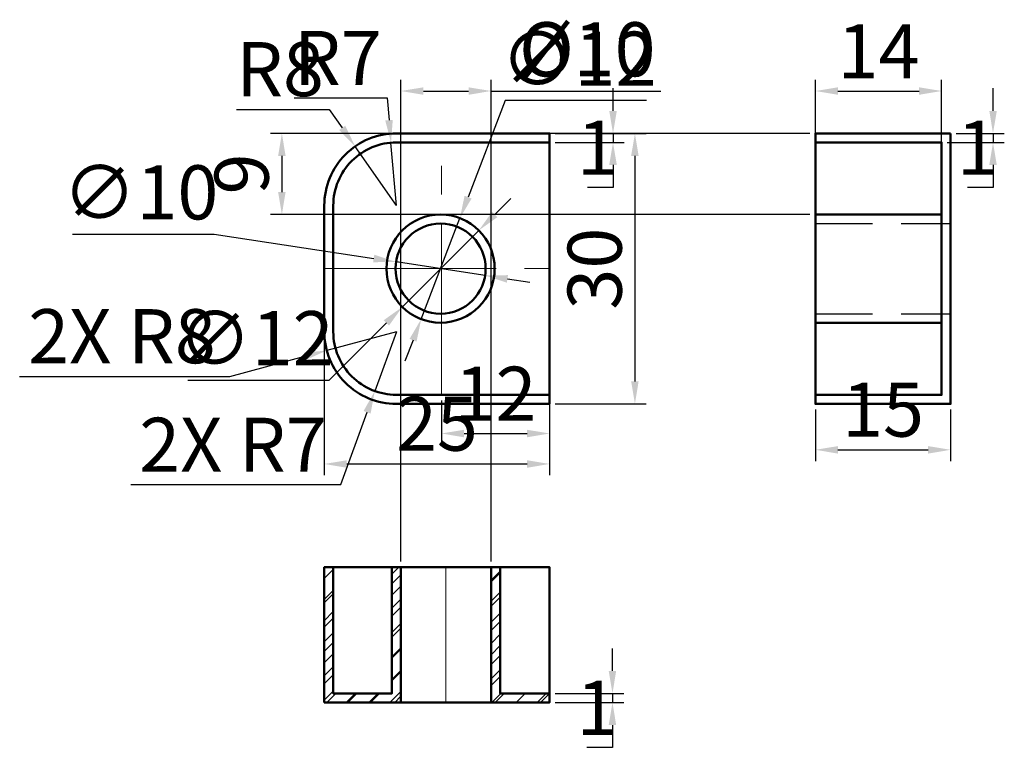
# Model space of a CAD drawing. Units: millimetres. Extents: x 12 to 121, y 26 to 107.
import ezdxf

# ---------------------------------------------------------------- set-up
doc = ezdxf.new("R2010")
doc.units = ezdxf.units.MM
doc.linetypes.add('CENTER2', pattern=[28.575, 19.05, -3.175, 3.175, -3.175])
doc.linetypes.add('HIDDEN', pattern=[9.525, 6.35, -3.175])
for name, color, linetype, lineweight in [('M-CNTR', 1, 'CENTER2', 18), ('M-DIMS', 2, 'Continuous', 25), ('M-HATC', 8, 'Continuous', 18), ('M-HIDN', 3, 'HIDDEN', 25), ('M-OUTL', 7, 'Continuous', 50)]:
    doc.layers.add(name, color=color, linetype=linetype, lineweight=lineweight)
doc.styles.get("Standard").update_dxf_attribs({"font": 'arial.ttf'})
doc.dimstyles.new('ISO-25', dxfattribs={"dimtxt": 6, "dimasz": 2.5, "dimexe": 1.25, "dimexo": 0.625, "dimtad": 1, "dimtoh": 1, "dimdec": 0, "dimtxsty": 'Standard', "dimcen": 2.5, "dimadec": 0, "dimazin": 0, "dimtfac": 1, "dimtdec": 0, "dimtmove": 0, "dimatfit": 3, "dimfxl": 1, "dimarcsym": 0})

# ---------------------------------------------------------------- blocks, each defined once
blk = doc.blocks.new('*D1')
at = {"layer": 'Defpoints', "color": 0, "transparency": 16777216}
for p in [(70.42, 94.79), (70.42, 93.79), (77.45, 93.79)]:
    blk.add_point(p, dxfattribs=at)
at = {"layer": 'M-DIMS', "color": 0, "lineweight": -2, "transparency": 16777216}
for p, q in [((77.45, 97.29), (77.45, 99.79)), ((71.04, 94.79), (78.7, 94.79)), ((77.45, 94.79), (77.45, 93.79)), ((71.04, 93.79), (78.7, 93.79)), ((77.45, 91.29), (77.45, 88.79)), ((77.45, 88.79), (74.61, 88.79))]:
    blk.add_line(p, q, dxfattribs=at)
at = {"layer": 'M-DIMS', "color": 0, "transparency": 16777216}
for points in [[(77.03, 97.29), (77.87, 97.29), (77.45, 94.79)], [(77.03, 91.29), (77.87, 91.29), (77.45, 93.79)]]:
    blk.add_solid(points, dxfattribs=at)
at = {"layer": 'M-DIMS', "color": 0, "transparency": 16777216, "insert": (75.72, 92.42), "char_height": 6, "attachment_point": 5}
blk.add_mtext('1', dxfattribs=at)
blk = doc.blocks.new('*D2')
at = {"layer": 'Defpoints', "color": 0, "transparency": 16777216}
for p in [(70.42, 94.79), (70.42, 64.79), (79.88, 64.79)]:
    blk.add_point(p, dxfattribs=at)
at = {"layer": 'M-DIMS', "color": 0, "lineweight": -2, "transparency": 16777216}
for p, q in [((71.04, 94.79), (81.13, 94.79)), ((79.88, 92.29), (79.88, 67.29)), ((71.04, 64.79), (81.13, 64.79))]:
    blk.add_line(p, q, dxfattribs=at)
at = {"layer": 'M-DIMS', "color": 0, "transparency": 16777216}
for points in [[(79.46, 92.29), (80.29, 92.29), (79.88, 94.79)], [(79.46, 67.29), (80.29, 67.29), (79.88, 64.79)]]:
    blk.add_solid(points, dxfattribs=at)
at = {"layer": 'M-DIMS', "color": 0, "transparency": 16777216, "insert": (76.19, 79.79), "char_height": 6, "attachment_point": 5, "rotation": 90}
blk.add_mtext('30', dxfattribs=at)
blk = doc.blocks.new('*D3')
at = {"layer": 'Defpoints', "color": 0, "transparency": 16777216}
for p in [(48.84, 93.35), (53.42, 86.79)]:
    blk.add_point(p, dxfattribs=at)
at = {"layer": 'M-DIMS', "color": 0, "lineweight": -2, "transparency": 16777216}
for p, q in [((35.67, 97.45), (45.98, 97.45)), ((45.98, 97.45), (47.41, 95.4)), ((53.42, 86.79), (48.84, 93.35))]:
    blk.add_line(p, q, dxfattribs=at)
at = {"layer": 'M-DIMS', "color": 0, "transparency": 16777216}
blk.add_solid([(47.75, 95.64), (47.07, 95.16), (48.84, 93.35)], dxfattribs=at)
at = {"layer": 'M-DIMS', "color": 0, "transparency": 16777216, "insert": (40.51, 101.14), "char_height": 6, "attachment_point": 5}
blk.add_mtext('R8', dxfattribs=at)
blk = doc.blocks.new('*D4')
at = {"layer": 'Defpoints', "color": 0, "transparency": 16777216}
for p in [(52.82, 93.76), (53.42, 86.79)]:
    blk.add_point(p, dxfattribs=at)
at = {"layer": 'M-DIMS', "color": 0, "lineweight": -2, "transparency": 16777216}
for p, q in [((42.09, 98.74), (52.39, 98.74)), ((52.39, 98.74), (52.61, 96.25)), ((53.42, 86.79), (52.82, 93.76))]:
    blk.add_line(p, q, dxfattribs=at)
at = {"layer": 'M-DIMS', "color": 0, "transparency": 16777216}
blk.add_solid([(53.02, 96.29), (52.19, 96.22), (52.82, 93.76)], dxfattribs=at)
at = {"layer": 'M-DIMS', "color": 0, "transparency": 16777216, "insert": (46.93, 102.37), "char_height": 6, "attachment_point": 5}
blk.add_mtext('R7', dxfattribs=at)
blk = doc.blocks.new('*D5')
at = {"layer": 'Defpoints', "color": 0, "transparency": 16777216}
for p in [(58.42, 65.79), (70.42, 65.79), (70.42, 61.51)]:
    blk.add_point(p, dxfattribs=at)
at = {"layer": 'M-DIMS', "color": 0, "lineweight": -2, "transparency": 16777216}
for p, q in [((58.42, 65.16), (58.42, 60.26)), ((70.42, 65.16), (70.42, 60.26)), ((60.92, 61.51), (67.92, 61.51))]:
    blk.add_line(p, q, dxfattribs=at)
at = {"layer": 'M-DIMS', "color": 0, "transparency": 16777216}
for points in [[(60.92, 61.92), (60.92, 61.09), (58.42, 61.51)], [(67.92, 61.92), (67.92, 61.09), (70.42, 61.51)]]:
    blk.add_solid(points, dxfattribs=at)
at = {"layer": 'M-DIMS', "color": 0, "transparency": 16777216, "insert": (64.42, 65.14), "char_height": 6, "attachment_point": 5}
blk.add_mtext('12', dxfattribs=at)
blk = doc.blocks.new('*D6')
at = {"layer": 'Defpoints', "color": 0, "transparency": 16777216}
for p in [(45.42, 72.79), (70.42, 72.79), (70.42, 58.13)]:
    blk.add_point(p, dxfattribs=at)
at = {"layer": 'M-DIMS', "color": 0, "lineweight": -2, "transparency": 16777216}
for p, q in [((45.42, 72.16), (45.42, 56.88)), ((70.42, 72.16), (70.42, 56.88)), ((47.92, 58.13), (67.92, 58.13))]:
    blk.add_line(p, q, dxfattribs=at)
at = {"layer": 'M-DIMS', "color": 0, "transparency": 16777216}
for points in [[(47.92, 58.54), (47.92, 57.71), (45.42, 58.13)], [(67.92, 58.54), (67.92, 57.71), (70.42, 58.13)]]:
    blk.add_solid(points, dxfattribs=at)
at = {"layer": 'M-DIMS', "color": 0, "transparency": 16777216, "insert": (57.92, 61.82), "char_height": 6, "attachment_point": 5}
blk.add_mtext('25', dxfattribs=at)
blk = doc.blocks.new('*D7')
at = {"layer": 'Defpoints', "color": 0, "transparency": 16777216}
for p in [(99.9, 64.79), (114.9, 64.79), (114.9, 59.7)]:
    blk.add_point(p, dxfattribs=at)
at = {"layer": 'M-DIMS', "color": 0, "lineweight": -2, "transparency": 16777216}
for p, q in [((99.9, 64.16), (99.9, 58.45)), ((114.9, 64.16), (114.9, 58.45)), ((102.4, 59.7), (112.4, 59.7))]:
    blk.add_line(p, q, dxfattribs=at)
at = {"layer": 'M-DIMS', "color": 0, "transparency": 16777216}
for points in [[(102.4, 60.11), (102.4, 59.28), (99.9, 59.7)], [(112.4, 60.11), (112.4, 59.28), (114.9, 59.7)]]:
    blk.add_solid(points, dxfattribs=at)
at = {"layer": 'M-DIMS', "color": 0, "transparency": 16777216, "insert": (107.4, 63.38), "char_height": 6, "attachment_point": 5}
blk.add_mtext('15', dxfattribs=at)
blk = doc.blocks.new('*D8')
at = {"layer": 'Defpoints', "color": 0, "transparency": 16777216}
for p in [(60.47, 85.39), (56.17, 74.19)]:
    blk.add_point(p, dxfattribs=at)
at = {"layer": 'M-DIMS', "color": 0, "lineweight": -2, "transparency": 16777216}
for p, q in [((65.49, 98.44), (61.37, 87.72)), ((81.17, 98.44), (65.49, 98.44)), ((56.17, 74.19), (60.47, 85.39)), ((55.27, 71.85), (54.37, 69.52))]:
    blk.add_line(p, q, dxfattribs=at)
at = {"layer": 'M-DIMS', "color": 0, "transparency": 16777216}
for points in [[(60.98, 87.87), (61.76, 87.57), (60.47, 85.39)], [(54.88, 72), (55.66, 71.7), (56.17, 74.19)]]:
    blk.add_solid(points, dxfattribs=at)
at = {"layer": 'M-DIMS', "color": 0, "transparency": 16777216, "insert": (73.64, 102.29), "char_height": 6, "attachment_point": 5}
blk.add_mtext('∅12', dxfattribs=at)
blk = doc.blocks.new('*D9')
at = {"layer": 'Defpoints', "color": 0, "transparency": 16777216}
for p in [(53.38, 80.54), (63.26, 79.03)]:
    blk.add_point(p, dxfattribs=at)
at = {"layer": 'M-DIMS', "color": 0, "lineweight": -2, "transparency": 16777216}
for p, q in [((17.48, 83.61), (33.21, 83.61)), ((33.21, 83.61), (50.91, 80.92)), ((63.26, 79.03), (53.38, 80.54)), ((65.73, 78.66), (68.21, 78.28))]:
    blk.add_line(p, q, dxfattribs=at)
at = {"layer": 'M-DIMS', "color": 0, "transparency": 16777216}
for points in [[(50.97, 81.33), (50.84, 80.5), (53.38, 80.54)], [(65.8, 79.07), (65.67, 78.24), (63.26, 79.03)]]:
    blk.add_solid(points, dxfattribs=at)
at = {"layer": 'M-DIMS', "color": 0, "transparency": 16777216, "insert": (25.03, 87.47), "char_height": 6, "attachment_point": 5}
blk.add_mtext('∅10', dxfattribs=at)
blk = doc.blocks.new('*D10')
at = {"layer": 'Defpoints', "color": 0, "transparency": 16777216}
for p in [(70.42, 32.68), (70.42, 31.68), (77.39, 31.68)]:
    blk.add_point(p, dxfattribs=at)
at = {"layer": 'M-DIMS', "color": 0, "lineweight": -2, "transparency": 16777216}
for p, q in [((77.39, 35.18), (77.39, 37.68)), ((71.04, 32.68), (78.64, 32.68)), ((71.04, 31.68), (78.64, 31.68)), ((77.39, 32.68), (77.39, 31.68)), ((77.39, 29.18), (77.39, 26.68)), ((77.39, 26.68), (74.55, 26.68))]:
    blk.add_line(p, q, dxfattribs=at)
at = {"layer": 'M-DIMS', "color": 0, "transparency": 16777216}
for points in [[(76.97, 35.18), (77.8, 35.18), (77.39, 32.68)], [(76.97, 29.18), (77.8, 29.18), (77.39, 31.68)]]:
    blk.add_solid(points, dxfattribs=at)
at = {"layer": 'M-DIMS', "color": 0, "transparency": 16777216, "insert": (75.66, 30.31), "char_height": 6, "attachment_point": 5}
blk.add_mtext('1', dxfattribs=at)
blk = doc.blocks.new('*D11')
at = {"layer": 'Defpoints', "color": 0, "transparency": 16777216}
for p in [(63.92, 99.49), (53.92, 46.68), (63.92, 46.68)]:
    blk.add_point(p, dxfattribs=at)
at = {"layer": 'M-DIMS', "color": 0, "lineweight": -2, "transparency": 16777216}
for p, q in [((53.92, 47.3), (53.92, 100.74)), ((63.92, 47.3), (63.92, 100.74)), ((56.42, 99.49), (61.42, 99.49)), ((63.92, 99.49), (82.77, 99.49))]:
    blk.add_line(p, q, dxfattribs=at)
at = {"layer": 'M-DIMS', "color": 0, "transparency": 16777216}
for points in [[(56.42, 99.9), (56.42, 99.07), (53.92, 99.49)], [(61.42, 99.9), (61.42, 99.07), (63.92, 99.49)]]:
    blk.add_solid(points, dxfattribs=at)
at = {"layer": 'M-DIMS', "color": 0, "transparency": 16777216, "insert": (74.59, 103.34), "char_height": 6, "attachment_point": 5}
blk.add_mtext('%%c10', dxfattribs=at)
blk = doc.blocks.new('*D12')
at = {"layer": 'Defpoints', "color": 0, "transparency": 16777216}
for p in [(99.9, 94.79), (40.72, 85.79), (99.9, 85.79)]:
    blk.add_point(p, dxfattribs=at)
at = {"layer": 'M-DIMS', "color": 0, "lineweight": -2, "transparency": 16777216}
for p, q in [((99.28, 94.79), (39.47, 94.79)), ((40.72, 92.29), (40.72, 88.29)), ((99.28, 85.79), (39.47, 85.79))]:
    blk.add_line(p, q, dxfattribs=at)
at = {"layer": 'M-DIMS', "color": 0, "transparency": 16777216}
for points in [[(40.3, 92.29), (41.13, 92.29), (40.72, 94.79)], [(40.3, 88.29), (41.13, 88.29), (40.72, 85.79)]]:
    blk.add_solid(points, dxfattribs=at)
at = {"layer": 'M-DIMS', "color": 0, "transparency": 16777216, "insert": (37.03, 90.29), "char_height": 6, "attachment_point": 5, "rotation": 90}
blk.add_mtext('9', dxfattribs=at)
blk = doc.blocks.new('*D13')
at = {"layer": 'Defpoints', "color": 0, "transparency": 16777216}
for p in [(113.9, 99.49), (99.9, 85.79), (113.9, 85.79)]:
    blk.add_point(p, dxfattribs=at)
at = {"layer": 'M-DIMS', "color": 0, "lineweight": -2, "transparency": 16777216}
for p, q in [((99.9, 86.41), (99.9, 100.74)), ((113.9, 86.41), (113.9, 100.74)), ((102.4, 99.49), (111.4, 99.49))]:
    blk.add_line(p, q, dxfattribs=at)
at = {"layer": 'M-DIMS', "color": 0, "transparency": 16777216}
for points in [[(102.4, 99.9), (102.4, 99.07), (99.9, 99.49)], [(111.4, 99.9), (111.4, 99.07), (113.9, 99.49)]]:
    blk.add_solid(points, dxfattribs=at)
at = {"layer": 'M-DIMS', "color": 0, "transparency": 16777216, "insert": (106.9, 103.12), "char_height": 6, "attachment_point": 5}
blk.add_mtext('14', dxfattribs=at)
blk = doc.blocks.new('*D14')
at = {"layer": 'Defpoints', "color": 0, "transparency": 16777216}
for p in [(114.9, 94.79), (113.9, 93.79), (119.6, 93.79)]:
    blk.add_point(p, dxfattribs=at)
at = {"layer": 'M-DIMS', "color": 0, "lineweight": -2, "transparency": 16777216}
for p, q in [((119.6, 97.29), (119.6, 99.79)), ((115.53, 94.79), (120.85, 94.79)), ((119.6, 94.79), (119.6, 93.79)), ((114.53, 93.79), (120.85, 93.79)), ((119.6, 91.29), (119.6, 88.79)), ((119.6, 88.79), (116.77, 88.79))]:
    blk.add_line(p, q, dxfattribs=at)
at = {"layer": 'M-DIMS', "color": 0, "transparency": 16777216}
for points in [[(119.19, 97.29), (120.02, 97.29), (119.6, 94.79)], [(119.19, 91.29), (120.02, 91.29), (119.6, 93.79)]]:
    blk.add_solid(points, dxfattribs=at)
at = {"layer": 'M-DIMS', "color": 0, "transparency": 16777216, "insert": (117.87, 92.42), "char_height": 6, "attachment_point": 5}
blk.add_mtext('1', dxfattribs=at)
blk = doc.blocks.new('*D15')
at = {"layer": 'Defpoints', "color": 0, "transparency": 16777216}
for p in [(62.56, 84.03), (54.08, 75.54)]:
    blk.add_point(p, dxfattribs=at)
at = {"layer": 'M-DIMS', "color": 0, "lineweight": -2, "transparency": 16777216}
for p, q in [((64.33, 85.8), (66.1, 87.56)), ((62.56, 84.03), (54.08, 75.54)), ((45.97, 67.44), (52.31, 73.78)), ((30.28, 67.44), (45.97, 67.44))]:
    blk.add_line(p, q, dxfattribs=at)
at = {"layer": 'M-DIMS', "color": 0, "transparency": 16777216}
for points in [[(64.04, 86.09), (64.62, 85.5), (62.56, 84.03)], [(52.01, 74.07), (52.6, 73.48), (54.08, 75.54)]]:
    blk.add_solid(points, dxfattribs=at)
at = {"layer": 'M-DIMS', "color": 0, "transparency": 16777216, "insert": (37.82, 71.3), "char_height": 6, "attachment_point": 5}
blk.add_mtext('∅12', dxfattribs=at)
blk = doc.blocks.new('*D16')
at = {"layer": 'Defpoints', "color": 0, "transparency": 16777216}
for p in [(53.42, 72.79), (45.69, 70.71)]:
    blk.add_point(p, dxfattribs=at)
at = {"layer": 'M-DIMS', "color": 0, "lineweight": -2, "transparency": 16777216}
for p, q in [((53.42, 72.79), (45.69, 70.71)), ((34.94, 67.83), (43.27, 70.07)), ((11.63, 67.83), (34.94, 67.83))]:
    blk.add_line(p, q, dxfattribs=at)
at = {"layer": 'M-DIMS', "color": 0, "transparency": 16777216}
blk.add_solid([(43.17, 70.47), (43.38, 69.67), (45.69, 70.71)], dxfattribs=at)
at = {"layer": 'M-DIMS', "color": 0, "transparency": 16777216, "insert": (22.98, 71.52), "char_height": 6, "attachment_point": 5}
blk.add_mtext('2X R8', dxfattribs=at)
blk = doc.blocks.new('*D17')
at = {"layer": 'Defpoints', "color": 0, "transparency": 16777216}
for p in [(53.42, 72.79), (51.02, 66.21)]:
    blk.add_point(p, dxfattribs=at)
at = {"layer": 'M-DIMS', "color": 0, "lineweight": -2, "transparency": 16777216}
for p, q in [((53.42, 72.79), (51.02, 66.21)), ((47.25, 55.84), (50.17, 63.86)), ((23.96, 55.84), (47.25, 55.84))]:
    blk.add_line(p, q, dxfattribs=at)
at = {"layer": 'M-DIMS', "color": 0, "transparency": 16777216}
blk.add_solid([(49.78, 64), (50.56, 63.72), (51.02, 66.21)], dxfattribs=at)
at = {"layer": 'M-DIMS', "color": 0, "transparency": 16777216, "insert": (35.29, 59.48), "char_height": 6, "attachment_point": 5}
blk.add_mtext('2X R7', dxfattribs=at)

msp = doc.modelspace()

# ---------------------------------------------------------------- hatches: boundary and pattern name
at = {"layer": 'M-HATC'}
h = msp.add_hatch(dxfattribs=at)
h.set_pattern_fill('ANSI31', color=256, scale=0.6)
h.paths.add_polyline_path([(46.42, 46.68), (45.42, 46.68), (45.42, 31.68), (53.92, 31.68), (53.92, 46.68), (52.92, 46.68), (52.92, 32.68), (46.42, 32.68)])
h.paths.add_polyline_path([(64.92, 46.68), (63.92, 46.68), (63.92, 31.68), (70.42, 31.68), (70.42, 32.68), (64.92, 32.68)])
h = msp.add_hatch(dxfattribs=at)
h.set_pattern_fill('ANSI31', color=256, scale=0.52)
h.paths.add_polyline_path([(46.42, 46.68), (45.42, 46.68), (45.42, 31.68), (53.92, 31.68), (53.92, 46.68), (52.92, 46.68), (52.92, 32.68), (46.42, 32.68)])
h.paths.add_polyline_path([(64.92, 46.68), (63.92, 46.68), (63.92, 31.68), (70.42, 31.68), (70.42, 32.68), (64.92, 32.68)])

# ---------------------------------------------------------------- linework, layer by layer
at = {"layer": 'M-CNTR'}
for p, q in [((58.42, 65.79), (58.42, 93.79)), ((45.42, 79.79), (70.42, 79.79)), ((58.92, 46.68), (58.92, 31.68))]:
    msp.add_line(p, q, dxfattribs=at)
at = {"layer": 'M-HIDN'}
for p, q in [((99.9, 84.79), (114.9, 84.79)), ((99.9, 74.79), (114.9, 74.79))]:
    msp.add_line(p, q, dxfattribs=at)
at = {"layer": 'M-OUTL'}
for p, q in [((99.9, 85.79), (113.9, 85.79)), ((99.9, 73.79), (113.9, 73.79)), ((53.92, 46.68), (53.92, 31.68)), ((63.92, 46.68), (63.92, 31.68))]:
    msp.add_line(p, q, dxfattribs=at)
msp.add_lwpolyline([(70.42, 64.79), (70.42, 94.79), (53.42, 94.79, 0.414214), (45.42, 86.79), (45.42, 72.79, 0.414214), (53.42, 64.79)], format="xyb", close=True, dxfattribs=at)
for points in [[(114.9, 94.79), (114.9, 64.79), (99.9, 64.79), (99.9, 94.79)], [(45.42, 31.68), (70.42, 31.68), (70.42, 46.68), (45.42, 46.68)]]:
    msp.add_lwpolyline(points, close=True, dxfattribs=at)
msp.add_lwpolyline([(70.42, 93.79), (53.42, 93.79, 0.414214), (46.42, 86.79), (46.42, 72.79, 0.414214), (53.42, 65.79), (70.42, 65.79)], format="xyb", dxfattribs=at)
for points in [[(99.9, 93.79), (113.9, 93.79), (113.9, 65.79), (99.9, 65.79)], [(52.92, 46.68), (52.92, 32.68), (46.42, 32.68), (46.42, 46.68)], [(64.92, 46.68), (64.92, 32.68), (70.42, 32.68)]]:
    msp.add_lwpolyline(points, dxfattribs=at)
for radius in [6, 5]:
    msp.add_circle((58.32, 79.79), radius, dxfattribs=at)

# ---------------------------------------------------------------- dimensions: what is measured, and where the dimension line sits
at = {"layer": 'M-DIMS'}
dim = msp.add_linear_dim(base=(63.92, 99.49), p1=(53.92, 46.68), p2=(63.92, 46.68), text='%%c<>', dimstyle='ISO-25', override={"dimdec": 0, "dimlfac": 1, "dimrnd": 0, "dimzin": 0, "dimdsep": 46, "dimlunit": 2}, dxfattribs=at)
dim.commit()
dim.dimension.update_dxf_attribs({"geometry": '*D11', "text_midpoint": (74.59, 103.34)})
for base, p1, p2, override, picture, middle in [((113.9, 99.49), (99.9, 85.79), (113.9, 85.79), {"dimdec": 0, "dimlfac": 1, "dimrnd": 0, "dimzin": 0, "dimdsep": 46, "dimlunit": 2}, '*D13', (106.9, 103.12)), ((70.42, 58.13), (45.42, 72.79), (70.42, 72.79), {"dimclrd": 0, "dimclre": 0, "dimclrt": 0}, '*D6', (57.92, 61.82)), ((70.42, 61.51), (58.42, 65.79), (70.42, 65.79), {"dimclrd": 0, "dimclre": 0, "dimclrt": 0}, '*D5', (64.42, 65.14)), ((114.9, 59.7), (99.9, 64.79), (114.9, 64.79), {"dimclrd": 0, "dimclre": 0, "dimclrt": 0}, '*D7', (107.4, 63.38))]:
    dim = msp.add_linear_dim(base=base, p1=p1, p2=p2, dimstyle='ISO-25', override=override, dxfattribs=at)
    dim.commit()
    dim.dimension.update_dxf_attribs({"geometry": picture, "text_midpoint": middle})
for mpoint, picture, middle in [((52.82, 93.76), '*D4', (46.93, 102.37)), ((48.84, 93.35), '*D3', (40.51, 101.14))]:
    dim = msp.add_radius_dim(center=(53.42, 86.79), mpoint=mpoint, dimstyle='ISO-25', override={"dimclrd": 0, "dimclre": 0, "dimclrt": 0}, dxfattribs=at)
    dim.commit()
    dim.dimension.update_dxf_attribs({"geometry": picture, "text_midpoint": middle})
for p1, p2, override, picture, middle in [((56.17, 74.19), (60.47, 85.39), {"dimclrd": 0, "dimclre": 0, "dimclrt": 0}, '*D8', (73.64, 98.44)), ((63.26, 79.03), (53.38, 80.54), {"dimclrd": 0, "dimclre": 0, "dimclrt": 0}, '*D9', (33.21, 83.61)), ((62.56, 84.03), (54.08, 75.54), {"dimdec": 0, "dimlfac": 1, "dimrnd": 0, "dimzin": 0, "dimdsep": 46, "dimlunit": 2}, '*D15', (37.82, 67.44))]:
    dim = msp.add_diameter_dim_2p(p1=p1, p2=p2, dimstyle='ISO-25', override=override, dxfattribs=at)
    dim.commit()
    dim.dimension.update_dxf_attribs({"geometry": picture, "text_midpoint": middle, "dimtype": 163})
for base, p1, p2, override, picture, middle in [((77.45, 93.79), (70.42, 94.79), (70.42, 93.79), {"dimclrd": 0, "dimclre": 0, "dimclrt": 0}, '*D1', (75.72, 92.42)), ((119.6, 93.79), (114.9, 94.79), (113.9, 93.79), {"dimdec": 0, "dimlfac": 1, "dimrnd": 0, "dimzin": 0, "dimdsep": 46, "dimlunit": 2}, '*D14', (117.87, 92.42)), ((40.72, 85.79), (99.9, 94.79), (99.9, 85.79), {"dimdec": 0, "dimlfac": 1, "dimrnd": 0, "dimzin": 0, "dimdsep": 46, "dimlunit": 2}, '*D12', (37.03, 90.29)), ((79.88, 64.79), (70.42, 94.79), (70.42, 64.79), {"dimclrd": 0, "dimclre": 0, "dimclrt": 0}, '*D2', (76.19, 79.79)), ((77.39, 31.68), (70.42, 32.68), (70.42, 31.68), {"dimclrd": 0, "dimclre": 0, "dimclrt": 0}, '*D10', (75.66, 30.31))]:
    dim = msp.add_linear_dim(base=base, p1=p1, p2=p2, angle=90, dimstyle='ISO-25', override=override, dxfattribs=at)
    dim.commit()
    dim.dimension.update_dxf_attribs({"geometry": picture, "text_midpoint": middle})
for mpoint, picture, middle in [((45.69, 70.71), '*D16', (22.98, 71.52)), ((51.02, 66.21), '*D17', (35.29, 59.48))]:
    dim = msp.add_radius_dim(center=(53.42, 72.79), mpoint=mpoint, text='2X <>', dimstyle='ISO-25', override={"dimdec": 0, "dimlfac": 1, "dimrnd": 0, "dimzin": 0, "dimdsep": 46, "dimlunit": 2}, dxfattribs=at)
    dim.commit()
    dim.dimension.update_dxf_attribs({"geometry": picture, "text_midpoint": middle})

doc.saveas('drawing.dxf')
